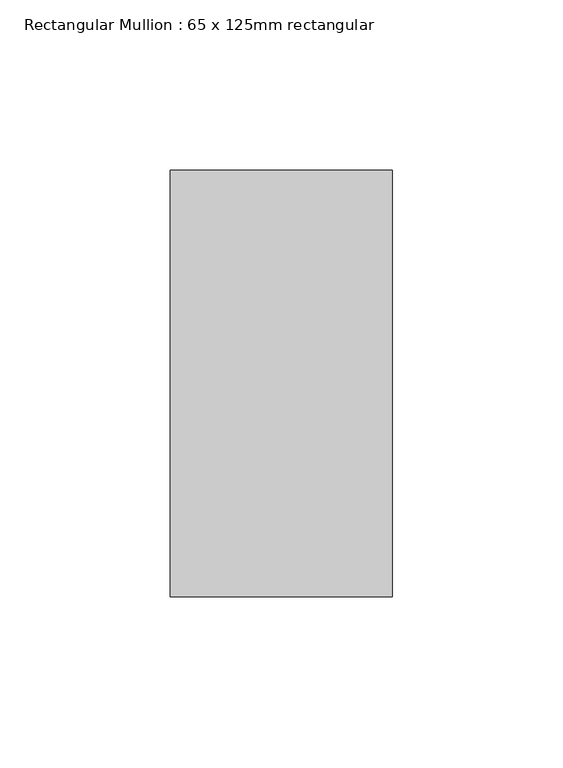
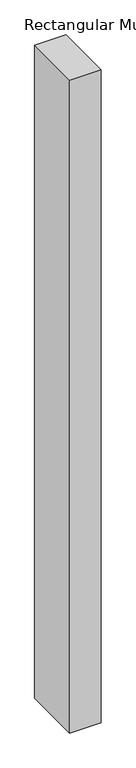
"""IFC4 building model written with IfcOpenShell, lengths in millimetres: member geometry, Rectangular Mullion : 65 x 125mm rectangular."""

from ifc_helpers import new_model, si_unit, frame, origin, place, context, project, spatial, polyline, outline, extrude, source, transform, mapped, element, save


def rectangular_mullion_65_x_125mm_rectangular_f4cebacc(model_context):
    return source(origin(), model_context, "Body", "SweptSolid", [
        extrude(outline(polyline([(0.0, 62.5), (0.0, -62.5), (-65.0, -62.5), (-65.0, 62.5), (0.0, 62.5)])), frame((0.0, 0.0, -1425.0), z_axis=(0.0, 0.0, 1.0), x_axis=(1.0, 0.0, 0.0)), (0.0, 0.0, 1.0), 1425.0),
    ])


if __name__ == "__main__":
    model = new_model("IFC4")
    model_context = context("Model", 3, world=origin())
    ifc_project = project(units=[si_unit("LENGTHUNIT", "METRE", prefix="MILLI")], contexts=[model_context])
    site = spatial("IfcSite", under=ifc_project)
    building = spatial("IfcBuilding", under=site)
    placement = place(None, origin())
    rectangular_mullion_65_x_125mm_rectangular_shape = rectangular_mullion_65_x_125mm_rectangular_f4cebacc(model_context)
    element("IfcMember", 1, ObjectType="Rectangular Mullion : 65 x 125mm rectangular", at=placement, inside=building, context=model_context, shape_type="MappedRepresentation", body=[
        mapped(rectangular_mullion_65_x_125mm_rectangular_shape, transform((0.0, 0.0, 0.0), x_axis=(1.0, 0.0, 0.0), y_axis=(0.0, 1.0, 0.0), z_axis=(0.0, 0.0, 1.0))),
    ])
    save(model, "model.ifc")

# Revit data of these elements
# Type "Rectangular Mullion : 65 x 125mm rectangular"
#   built-in parameter 1007304 = 0.410105 (stored number, unit not read)
#   built-in parameter 1007301 = 0.106627 (stored number, unit not read)
#   built-in parameter 1007300 = 0.106627 (stored number, unit not read)
# Element 1 (IfcMember, "Rectangular Mullion : 65 x 125mm rectangular")
#   Materials on its faces: "Aluminum"
# Materials
#   "Aluminum": class "Metal", colour RGB 244 245 246, transparency 0, Description = "Aluminum 6061", Cost = 0
